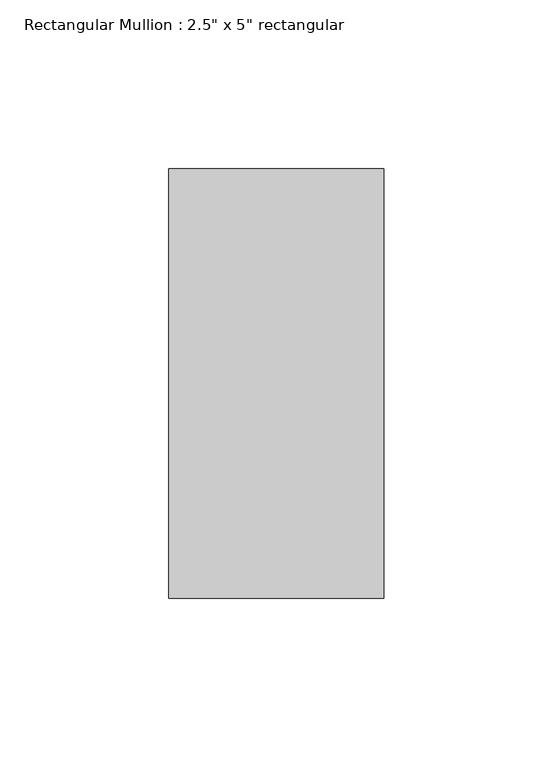
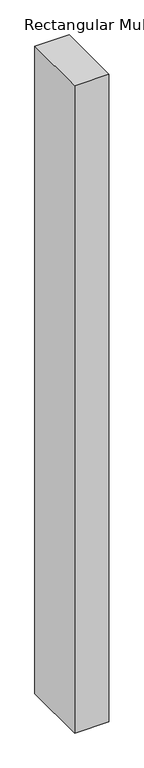
"""IFC4 building model written with IfcOpenShell, lengths in millimetres: member geometry."""

from ifc_helpers import new_model, si_unit, frame, origin, place, context, project, spatial, polyline, outline, extrude, source, transform, mapped, element, save


def member_2af3cda3(model_context):
    return source(origin(), model_context, "Body", "SweptSolid", [
        extrude(outline(polyline([(0.0, 63.5), (0.0, -63.5), (-63.5, -63.5), (-63.5, 63.5), (0.0, 63.5)])), frame((0.0, 0.0, -1264.0647091), z_axis=(0.0, 0.0, 1.0), x_axis=(1.0, 0.0, 0.0)), (0.0, 0.0, 1.0), 1264.0647091),
    ])


if __name__ == "__main__":
    model = new_model("IFC4")
    model_context = context("Model", 3, world=origin())
    ifc_project = project(units=[si_unit("LENGTHUNIT", "METRE", prefix="MILLI")], contexts=[model_context])
    site = spatial("IfcSite", under=ifc_project)
    building = spatial("IfcBuilding", under=site)
    placement = place(None, origin())
    member_shape = member_2af3cda3(model_context)
    element("IfcMember", 1, ObjectType="Rectangular Mullion : 2.5\" x 5\" rectangular", at=placement, inside=building, context=model_context, shape_type="MappedRepresentation", body=[
        mapped(member_shape, transform((0.0, 0.0, 0.0), x_axis=(1.0, 0.0, 0.0), y_axis=(0.0, 1.0, 0.0), z_axis=(0.0, 0.0, 1.0))),
    ])
    save(model, "model.ifc")

# Revit data of these elements
# Type "Rectangular Mullion : 2.5\" x 5\" rectangular"
#   built-in parameter 1007304 = 0.416667 (stored number, unit not read)
#   built-in parameter 1007301 = 0.104167 (stored number, unit not read)
#   built-in parameter 1007300 = 0.104167 (stored number, unit not read)
